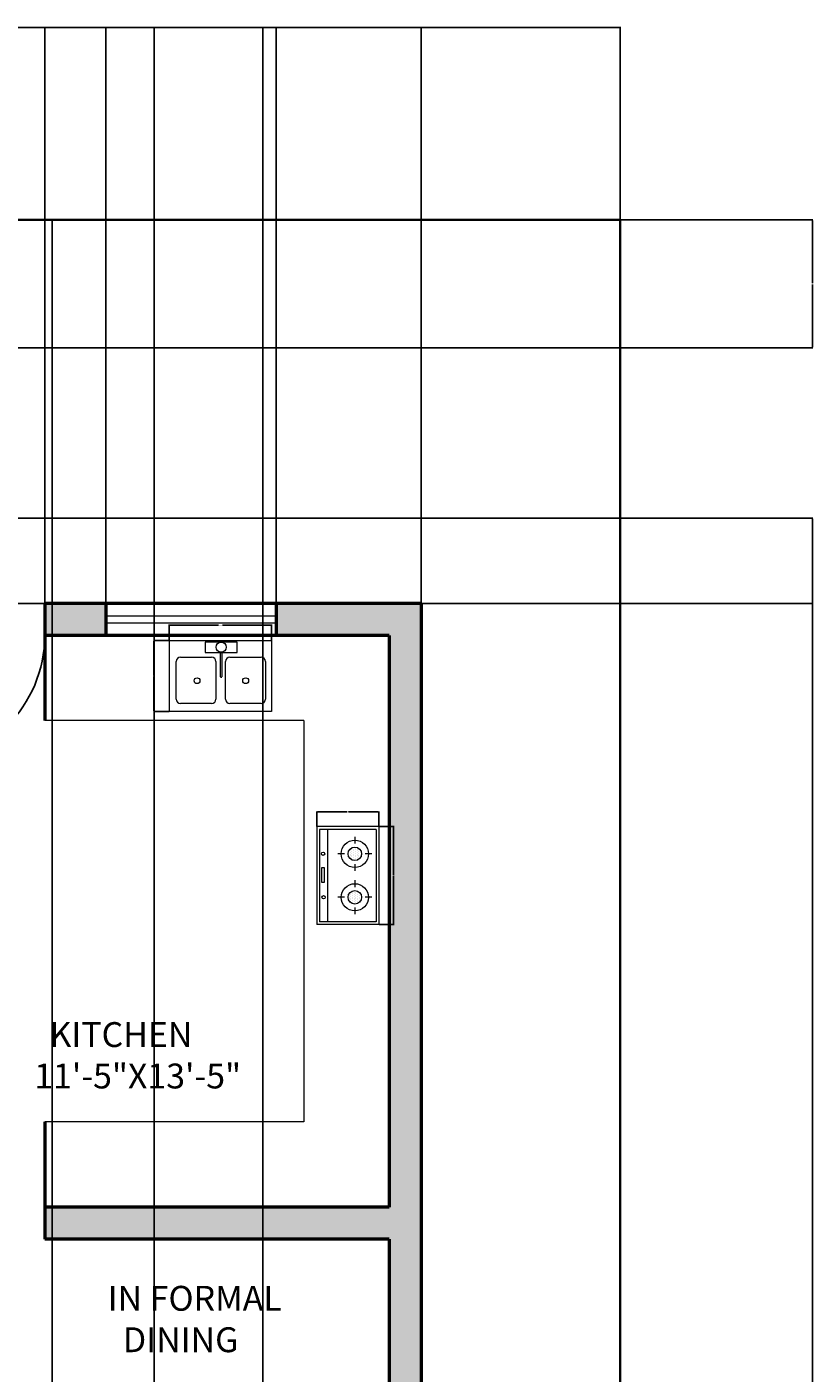
# Model space of a CAD drawing. Units: inches. Extents: x 2447 to 3157, y 2799 to 3988.
# Tile 9 of 9: x 2935 to 3157, y 3609 to 3988. Entities that reach past the tile are written whole.
import ezdxf

# ---------------------------------------------------------------- set-up
doc = ezdxf.new("R2010")
doc.units = ezdxf.units.IN
for name, color, linetype, lineweight in [('A-ANNO-DIMS', 2, 'Continuous', 18), ('A-AREA-IDEN', 7, 'Continuous', 25), ('A-DOOR', 3, 'Continuous', 25), ('A-EQPM', 8, 'Continuous', 18), ('A-FLOR-CASE', 8, 'Continuous', 20), ('A-FLOR-FIXT', 9, 'Continuous', 18), ('A-FLOR-STRS', 7, 'Continuous', 25), ('A-GLAZ', 4, 'Continuous', 18), ('A-WALL', 7, 'Continuous', 50), ('A-WALL-PATT', 252, 'Continuous', 13), ('C-PROP', 6, 'Continuous', 35)]:
    doc.layers.add(name, color=color, linetype=linetype, lineweight=lineweight)
doc.styles.get("Standard").update_dxf_attribs({"font": 'arial.ttf'})
doc.dimstyles.get("Standard").update_dxf_attribs({"dimtxt": 0.18, "dimasz": 0.18, "dimexe": 0.18, "dimexo": 0.0625, "dimgap": 0.09, "dimtad": 0, "dimtih": 1, "dimtoh": 1, "dimdec": 4, "dimzin": 0, "dimdsep": 46, "dimtxsty": 'Standard', "dimcen": 0.09, "dimadec": 0, "dimazin": 0, "dimtfac": 1, "dimtdec": 4, "dimtofl": 0, "dimtmove": 0, "dimatfit": 3, "dimfxl": 1, "dimtolj": 1, "dimtzin": 0, "dimarcsym": 0})

# ---------------------------------------------------------------- blocks, each defined once
blk = doc.blocks.new('A$C3AD04490')
for p, q in [((0, 641), (0, 0)), ((0, 641), (925, 641)), ((614, 627), (323, 627)), ((323, 627), (323, 532)), ((614, 532), (614, 627)), ((925, 641), (925, 0)), ((101, 490), (383, 490)), ((323, 532), (614, 532)), ((463, 312), (463, 537)), ((474, 537), (474, 312)), ((548, 490), (830, 490)), ((62, 111), (62, 451)), ((422, 451), (422, 111)), ((509, 111), (509, 451)), ((869, 451), (869, 111)), ((463, 311), (474, 311)), ((383, 72), (101, 72)), ((830, 72), (548, 72)), ((925, 0), (0, 0))]:
    blk.add_line(p, q)
for centre, radius in [((469, 581), 45.9), ((251, 278), 26.4), ((691, 278), 26.4)]:
    blk.add_circle(centre, radius)
for centre, start, end in [((101, 451), 90, 180), ((383, 451), 0, 90), ((548, 451), 90, 180), ((830, 451), 0, 90), ((101, 111), 180, 270), ((383, 111), 270, 0), ((548, 111), 180, 270), ((830, 111), 270, 0)]:
    blk.add_arc(centre, 39.1, start, end)
blk = doc.blocks.new('A$C475E21CF')
for p, q in [((0, 444.5), (0, 0)), ((0, 444.5), (699.9, 444.5)), ((19.4, 425), (19.4, 19.4)), ((19.4, 425), (680.5, 425)), ((194.5, 393.9), (194.5, 345.2)), ((505.4, 393.9), (505.4, 345.2)), ((680.5, 425), (680.5, 19.4)), ((699.9, 444.5), (699.9, 0)), ((166.9, 300.5), (166.9, 300.5)), ((179.1, 300.5), (179.1, 300.5)), ((185.2, 312.7), (185.2, 312.7)), ((191.2, 300.5), (191.2, 300.5)), ((197.3, 312.7), (197.3, 312.7)), ((203.4, 300.5), (203.4, 300.5)), ((209.5, 312.7), (209.5, 312.7)), ((215.6, 300.5), (215.6, 300.5)), ((227.7, 300.5), (227.7, 300.5)), ((474.1, 292.3), (474.1, 292.3)), ((480.2, 304.5), (480.2, 304.5)), ((486.3, 292.3), (486.3, 292.3)), ((492.3, 304.5), (492.3, 304.5)), ((498.4, 316.6), (498.4, 316.6)), ((498.4, 292.3), (498.4, 292.3)), ((504.5, 304.5), (504.5, 304.5)), ((510.6, 316.6), (510.6, 316.6)), ((510.6, 292.3), (510.6, 292.3)), ((516.7, 304.5), (516.7, 304.5)), ((522.7, 316.6), (522.7, 316.6)), ((522.7, 292.3), (522.7, 292.3)), ((528.8, 304.5), (528.8, 304.5)), ((534.9, 292.3), (534.9, 292.3)), ((541, 304.5), (541, 304.5)), ((547, 292.3), (547, 292.3)), ((72.9, 272.3), (121.6, 272.3)), ((148.7, 264.1), (148.7, 264.1)), ((154.8, 276.2), (154.8, 276.2)), ((154.8, 251.9), (154.8, 251.9)), ((160.9, 288.4), (160.9, 288.4)), ((160.9, 264.1), (160.9, 264.1)), ((160.9, 239.8), (160.9, 239.8)), ((166.9, 276.2), (166.9, 276.2)), ((166.9, 251.9), (166.9, 251.9)), ((173, 288.4), (173, 288.4)), ((173, 264.1), (173, 264.1)), ((173, 239.8), (173, 239.8)), ((179.1, 276.2), (179.1, 276.2)), ((179.1, 251.9), (179.1, 251.9)), ((179.1, 227.6), (179.1, 227.6)), ((185.2, 288.4), (185.2, 288.4)), ((185.2, 264.1), (185.2, 264.1)), ((185.2, 239.8), (185.2, 239.8)), ((191.2, 276.2), (191.2, 276.2)), ((191.2, 251.9), (191.2, 251.9)), ((191.2, 227.6), (191.2, 227.6)), ((194.5, 199.4), (194.5, 150.8)), ((197.3, 288.4), (197.3, 288.4)), ((197.3, 264.1), (197.3, 264.1)), ((197.3, 239.8), (197.3, 239.8)), ((203.4, 276.2), (203.4, 276.2)), ((203.4, 251.9), (203.4, 251.9)), ((203.4, 227.6), (203.4, 227.6)), ((209.5, 288.4), (209.5, 288.4)), ((209.5, 264.1), (209.5, 264.1)), ((209.5, 239.8), (209.5, 239.8)), ((215.6, 276.2), (215.6, 276.2)), ((215.6, 251.9), (215.6, 251.9)), ((215.6, 227.6), (215.6, 227.6)), ((221.6, 288.4), (221.6, 288.4)), ((221.6, 264.1), (221.6, 264.1)), ((221.6, 239.8), (221.6, 239.8)), ((227.7, 276.2), (227.7, 276.2)), ((227.7, 251.9), (227.7, 251.9)), ((233.8, 288.4), (233.8, 288.4)), ((233.8, 264.1), (233.8, 264.1)), ((233.8, 239.8), (233.8, 239.8)), ((239.9, 276.2), (239.9, 276.2)), ((239.9, 251.9), (239.9, 251.9)), ((267.4, 272.3), (316, 272.3)), ((383.9, 272.3), (432.5, 272.3)), ((462, 268), (462, 268)), ((468, 280.2), (468, 280.2)), ((468, 255.9), (468, 255.9)), ((474.1, 268), (474.1, 268)), ((474.1, 243.7), (474.1, 243.7)), ((480.2, 280.2), (480.2, 280.2)), ((480.2, 255.9), (480.2, 255.9)), ((486.3, 268), (486.3, 268)), ((486.3, 243.7), (486.3, 243.7)), ((492.3, 280.2), (492.3, 280.2)), ((492.3, 255.9), (492.3, 255.9)), ((492.3, 231.5), (492.3, 231.5)), ((498.4, 268), (498.4, 268)), ((498.4, 243.7), (498.4, 243.7)), ((504.5, 280.2), (504.5, 280.2)), ((504.5, 255.9), (504.5, 255.9)), ((504.5, 231.5), (504.5, 231.5)), ((505.4, 199.4), (505.4, 150.8)), ((510.6, 268), (510.6, 268)), ((510.6, 243.7), (510.6, 243.7)), ((516.7, 280.2), (516.7, 280.2)), ((516.7, 255.9), (516.7, 255.9)), ((516.7, 231.5), (516.7, 231.5)), ((522.7, 268), (522.7, 268)), ((522.7, 243.7), (522.7, 243.7)), ((528.8, 280.2), (528.8, 280.2)), ((528.8, 255.9), (528.8, 255.9)), ((528.8, 231.5), (528.8, 231.5)), ((534.9, 268), (534.9, 268)), ((534.9, 243.7), (534.9, 243.7)), ((541, 280.2), (541, 280.2)), ((541, 255.9), (541, 255.9)), ((547, 268), (547, 268)), ((547, 243.7), (547, 243.7)), ((553.1, 280.2), (553.1, 280.2)), ((553.1, 255.9), (553.1, 255.9)), ((578.4, 272.3), (627, 272.3)), ((0, 0), (699.9, 0)), ((19.4, 77.8), (680.5, 77.8)), ((19.4, 19.4), (680.5, 19.4)), ((293.4, 51.9), (400.6, 51.9)), ((293.4, 36.5), (293.4, 51.9)), ((400.6, 36.5), (293.4, 36.5)), ((400.6, 51.9), (400.6, 36.5))]:
    blk.add_line(p, q)
for centre, radius in [((194.5, 272.3), 97.2), ((194.5, 272.3), 48.6), ((505.4, 272.3), 97.2), ((505.4, 272.3), 48.6), ((193.9, 45.1), 11.7), ((505.2, 48.5), 11.7)]:
    blk.add_circle(centre, radius)
blk = doc.blocks.new('A$C1A936BB7')
blk.add_blockref('A$C475E21CF', (0, 0))
blk = doc.blocks.new('DOOR-SWING-36IN')
for p, q in [((0, 0), (0, 36)), ((1, 0), (1, 35.99)), ((1, 0), (0, 0))]:
    blk.add_line(p, q)
blk.add_arc((0, 0), 36, 0, 90)
blk = doc.blocks.new('*D30')
at = {"layer": 'A-ANNO-DIMS', "color": 0, "lineweight": -2, "transparency": 16777216}
for p, q in [((2975.45, 3815.28), (2975.45, 3819.71)), ((2975.63, 3819.53), (2989.29, 3819.53)), ((3004.04, 3819.53), (2990.38, 3819.53)), ((3004.22, 3815.28), (3004.22, 3819.71))]:
    blk.add_line(p, q, dxfattribs=at)
at = {"layer": 'A-ANNO-DIMS', "color": 0, "transparency": 16777216}
for points in [[(2975.63, 3819.56), (2975.63, 3819.5), (2975.45, 3819.53)], [(3004.04, 3819.56), (3004.04, 3819.5), (3004.22, 3819.53)]]:
    blk.add_solid(points, dxfattribs=at)
at = {"layer": 'Defpoints', "color": 0, "transparency": 16777216}
for p in [(3004.22, 3819.53), (2975.45, 3815.21), (3004.22, 3815.21)]:
    blk.add_point(p, dxfattribs=at)
at = {"layer": 'A-ANNO-DIMS', "color": 0, "transparency": 16777216, "insert": (2989.84, 3819.53), "char_height": 0.18, "attachment_point": 5}
blk.add_mtext('\\A1;SINK 29', dxfattribs=at)
blk = doc.blocks.new('*D31')
at = {"layer": 'A-ANNO-DIMS', "color": 0, "lineweight": -2, "transparency": 16777216}
for p, q in [((2975.39, 3815.21), (2970.95, 3815.21)), ((2971.13, 3815.03), (2971.13, 3805.43)), ((2971.13, 3795.46), (2971.13, 3805.07)), ((2975.39, 3795.28), (2970.95, 3795.28))]:
    blk.add_line(p, q, dxfattribs=at)
at = {"layer": 'A-ANNO-DIMS', "color": 0, "transparency": 16777216}
for points in [[(2971.1, 3815.03), (2971.16, 3815.03), (2971.13, 3815.21)], [(2971.1, 3795.46), (2971.16, 3795.46), (2971.13, 3795.28)]]:
    blk.add_solid(points, dxfattribs=at)
at = {"layer": 'Defpoints', "color": 0, "transparency": 16777216}
for p in [(2971.13, 3815.21), (2975.45, 3815.21), (2975.45, 3795.28)]:
    blk.add_point(p, dxfattribs=at)
at = {"layer": 'A-ANNO-DIMS', "color": 0, "transparency": 16777216, "insert": (2971.13, 3805.25), "char_height": 0.18, "attachment_point": 5}
blk.add_mtext('\\A1;20', dxfattribs=at)
blk = doc.blocks.new('*D32')
at = {"layer": 'A-ANNO-DIMS', "color": 0, "lineweight": -2, "transparency": 16777216}
for p, q in [((3034.53, 3762.83), (3038.78, 3762.83)), ((3038.6, 3762.65), (3038.6, 3749.24)), ((3038.6, 3735.46), (3038.6, 3748.87)), ((3034.53, 3735.28), (3038.78, 3735.28))]:
    blk.add_line(p, q, dxfattribs=at)
at = {"layer": 'A-ANNO-DIMS', "color": 0, "transparency": 16777216}
for points in [[(3038.57, 3762.65), (3038.63, 3762.65), (3038.6, 3762.83)], [(3038.57, 3735.46), (3038.63, 3735.46), (3038.6, 3735.28)]]:
    blk.add_solid(points, dxfattribs=at)
at = {"layer": 'Defpoints', "color": 0, "transparency": 16777216}
for p in [(3034.46, 3762.83), (3034.46, 3735.28), (3038.6, 3735.28)]:
    blk.add_point(p, dxfattribs=at)
at = {"layer": 'A-ANNO-DIMS', "color": 0, "transparency": 16777216, "insert": (3038.6, 3749.05), "char_height": 0.18, "attachment_point": 5}
blk.add_mtext('\\A1;HOB 28', dxfattribs=at)
blk = doc.blocks.new('*D33')
at = {"layer": 'A-ANNO-DIMS', "color": 0, "lineweight": -2, "transparency": 16777216}
for p, q in [((3016.96, 3762.89), (3016.96, 3767.14)), ((3017.14, 3766.96), (3025.5, 3766.96)), ((3034.28, 3766.96), (3025.92, 3766.96)), ((3034.46, 3762.89), (3034.46, 3767.14))]:
    blk.add_line(p, q, dxfattribs=at)
at = {"layer": 'A-ANNO-DIMS', "color": 0, "transparency": 16777216}
for points in [[(3017.14, 3766.99), (3017.14, 3766.93), (3016.96, 3766.96)], [(3034.28, 3766.99), (3034.28, 3766.93), (3034.46, 3766.96)]]:
    blk.add_solid(points, dxfattribs=at)
at = {"layer": 'Defpoints', "color": 0, "transparency": 16777216}
for p in [(3034.46, 3766.96), (3016.96, 3762.83), (3034.46, 3762.83)]:
    blk.add_point(p, dxfattribs=at)
at = {"layer": 'A-ANNO-DIMS', "color": 0, "transparency": 16777216, "insert": (3025.71, 3766.96), "char_height": 0.18, "attachment_point": 5}
blk.add_mtext('\\A1;17', dxfattribs=at)
blk = doc.blocks.new('*D46')
at = {"layer": 'A-ANNO-DIMS', "color": 0, "lineweight": -2, "transparency": 16777216}
for p, q in [((2561.37, 3849.76), (2561.37, 3988.03)), ((3046.37, 3825.76), (3046.37, 3988.03)), ((2561.55, 3987.85), (2803.57, 3987.85)), ((3046.19, 3987.85), (2804.16, 3987.85))]:
    blk.add_line(p, q, dxfattribs=at)
at = {"layer": 'A-ANNO-DIMS', "color": 0, "transparency": 16777216}
for points in [[(2561.55, 3987.88), (2561.55, 3987.82), (2561.37, 3987.85)], [(3046.19, 3987.88), (3046.19, 3987.82), (3046.37, 3987.85)]]:
    blk.add_solid(points, dxfattribs=at)
at = {"layer": 'Defpoints', "color": 0, "transparency": 16777216}
for p in [(3046.37, 3987.85), (2561.37, 3849.7), (3046.37, 3825.7)]:
    blk.add_point(p, dxfattribs=at)
at = {"layer": 'A-ANNO-DIMS', "color": 0, "transparency": 16777216, "insert": (2803.87, 3987.85), "char_height": 0.18, "attachment_point": 5}
blk.add_mtext('\\A1;485', dxfattribs=at)
blk = doc.blocks.new('*D47')
at = {"layer": 'A-ANNO-DIMS', "color": 0, "lineweight": -2, "transparency": 16777216}
for p, q in [((2798.43, 3849.7), (3156.7, 3849.7)), ((3156.52, 3849.52), (3156.52, 3487.38)), ((3156.52, 3124.88), (3156.52, 3487.02)), ((3046.43, 3124.7), (3156.7, 3124.7))]:
    blk.add_line(p, q, dxfattribs=at)
at = {"layer": 'A-ANNO-DIMS', "color": 0, "transparency": 16777216}
for points in [[(3156.49, 3849.52), (3156.55, 3849.52), (3156.52, 3849.7)], [(3156.49, 3124.88), (3156.55, 3124.88), (3156.52, 3124.7)]]:
    blk.add_solid(points, dxfattribs=at)
at = {"layer": 'Defpoints', "color": 0, "transparency": 16777216}
for p in [(2798.37, 3849.7), (3156.52, 3849.7), (3046.37, 3124.7)]:
    blk.add_point(p, dxfattribs=at)
at = {"layer": 'A-ANNO-DIMS', "color": 0, "transparency": 16777216, "insert": (3156.52, 3487.2), "char_height": 0.18, "attachment_point": 5}
blk.add_mtext('\\A1;725', dxfattribs=at)
blk = doc.blocks.new('*D49')
at = {"layer": 'A-ANNO-DIMS', "color": 0, "lineweight": -2, "transparency": 16777216}
for p, q in [((3046.37, 3825.76), (3046.37, 3988.03)), ((3102.37, 3933.76), (3102.37, 3988.03)), ((3046.55, 3987.85), (3074.15, 3987.85)), ((3102.19, 3987.85), (3074.59, 3987.85))]:
    blk.add_line(p, q, dxfattribs=at)
at = {"layer": 'A-ANNO-DIMS', "color": 0, "transparency": 16777216}
for points in [[(3046.55, 3987.88), (3046.55, 3987.82), (3046.37, 3987.85)], [(3102.19, 3987.88), (3102.19, 3987.82), (3102.37, 3987.85)]]:
    blk.add_solid(points, dxfattribs=at)
at = {"layer": 'Defpoints', "color": 0, "transparency": 16777216}
for p in [(3102.37, 3987.85), (3102.37, 3933.7), (3046.37, 3825.7)]:
    blk.add_point(p, dxfattribs=at)
at = {"layer": 'A-ANNO-DIMS', "color": 0, "transparency": 16777216, "insert": (3074.37, 3987.85), "char_height": 0.18, "attachment_point": 5}
blk.add_mtext('\\A1;56', dxfattribs=at)
blk = doc.blocks.new('*D50')
at = {"layer": 'A-ANNO-DIMS', "color": 0, "lineweight": -2, "transparency": 16777216}
for p, q in [((2832.46, 3897.64), (2832.46, 2799.37)), ((2942.46, 3897.64), (2942.46, 2799.37)), ((2832.64, 2799.55), (2887.18, 2799.55)), ((2942.28, 2799.55), (2887.74, 2799.55))]:
    blk.add_line(p, q, dxfattribs=at)
at = {"layer": 'A-ANNO-DIMS', "color": 0, "transparency": 16777216}
for points in [[(2832.64, 2799.58), (2832.64, 2799.52), (2832.46, 2799.55)], [(2942.28, 2799.58), (2942.28, 2799.52), (2942.46, 2799.55)]]:
    blk.add_solid(points, dxfattribs=at)
at = {"layer": 'Defpoints', "color": 0, "transparency": 16777216}
for p in [(2832.46, 3897.7), (2942.46, 3897.7), (2942.46, 2799.55)]:
    blk.add_point(p, dxfattribs=at)
at = {"layer": 'A-ANNO-DIMS', "color": 0, "transparency": 16777216, "insert": (2887.46, 2799.55), "char_height": 0.18, "attachment_point": 5}
blk.add_mtext('\\A1;110', dxfattribs=at)
blk = doc.blocks.new('*D51')
at = {"layer": 'A-ANNO-DIMS', "color": 0, "lineweight": -2, "transparency": 16777216}
for p, q in [((2942.52, 3933.7), (3156.7, 3933.7)), ((3156.52, 3933.52), (3156.52, 3915.88)), ((3156.52, 3897.88), (3156.52, 3915.52)), ((2942.52, 3897.7), (3156.7, 3897.7))]:
    blk.add_line(p, q, dxfattribs=at)
at = {"layer": 'A-ANNO-DIMS', "color": 0, "transparency": 16777216}
for points in [[(3156.49, 3933.52), (3156.55, 3933.52), (3156.52, 3933.7)], [(3156.49, 3897.88), (3156.55, 3897.88), (3156.52, 3897.7)]]:
    blk.add_solid(points, dxfattribs=at)
at = {"layer": 'Defpoints', "color": 0, "transparency": 16777216}
for p in [(2942.46, 3933.7), (3156.52, 3933.7), (2942.46, 3897.7)]:
    blk.add_point(p, dxfattribs=at)
at = {"layer": 'A-ANNO-DIMS', "color": 0, "transparency": 16777216, "insert": (3156.52, 3915.7), "char_height": 0.18, "attachment_point": 5}
blk.add_mtext('\\A1;36', dxfattribs=at)
blk = doc.blocks.new('*D62')
at = {"layer": 'A-ANNO-DIMS', "color": 0, "lineweight": -2, "transparency": 16777216}
for p, q in [((2798.43, 3849.7), (3156.7, 3849.7)), ((3156.52, 3849.52), (3156.52, 3837.88)), ((3156.52, 3825.88), (3156.52, 3837.52)), ((2798.43, 3825.7), (3156.7, 3825.7))]:
    blk.add_line(p, q, dxfattribs=at)
at = {"layer": 'A-ANNO-DIMS', "color": 0, "transparency": 16777216}
for points in [[(3156.49, 3849.52), (3156.55, 3849.52), (3156.52, 3849.7)], [(3156.49, 3825.88), (3156.55, 3825.88), (3156.52, 3825.7)]]:
    blk.add_solid(points, dxfattribs=at)
at = {"layer": 'Defpoints', "color": 0, "transparency": 16777216}
for p in [(2798.37, 3849.7), (2798.37, 3825.7), (3156.52, 3825.7)]:
    blk.add_point(p, dxfattribs=at)
at = {"layer": 'A-ANNO-DIMS', "color": 0, "transparency": 16777216, "insert": (3156.52, 3837.7), "char_height": 0.18, "attachment_point": 5}
blk.add_mtext('\\A1;24', dxfattribs=at)
blk = doc.blocks.new('*D65')
at = {"layer": 'A-ANNO-DIMS', "color": 0, "lineweight": -2, "transparency": 16777216}
for p, q in [((2940.37, 3825.76), (2940.37, 3988.03)), ((2957.58, 3825.76), (2957.58, 3988.03)), ((2940.55, 3987.85), (2948.52, 3987.85)), ((2957.4, 3987.85), (2949.43, 3987.85))]:
    blk.add_line(p, q, dxfattribs=at)
at = {"layer": 'A-ANNO-DIMS', "color": 0, "transparency": 16777216}
for points in [[(2940.55, 3987.88), (2940.55, 3987.82), (2940.37, 3987.85)], [(2957.4, 3987.88), (2957.4, 3987.82), (2957.58, 3987.85)]]:
    blk.add_solid(points, dxfattribs=at)
at = {"layer": 'Defpoints', "color": 0, "transparency": 16777216}
for p in [(2957.58, 3987.85), (2940.37, 3825.7), (2957.58, 3825.7)]:
    blk.add_point(p, dxfattribs=at)
at = {"layer": 'A-ANNO-DIMS', "color": 0, "transparency": 16777216, "insert": (2948.97, 3987.85), "char_height": 0.18, "attachment_point": 5}
blk.add_mtext('\\A1;17.213', dxfattribs=at)
blk = doc.blocks.new('*D66')
at = {"layer": 'A-ANNO-DIMS', "color": 0, "lineweight": -2, "transparency": 16777216}
for p, q in [((2957.58, 3825.76), (2957.58, 3988.03)), ((3005.58, 3825.76), (3005.58, 3988.03)), ((2957.76, 3987.85), (2981.36, 3987.85)), ((3005.4, 3987.85), (2981.8, 3987.85))]:
    blk.add_line(p, q, dxfattribs=at)
at = {"layer": 'A-ANNO-DIMS', "color": 0, "transparency": 16777216}
for points in [[(2957.76, 3987.88), (2957.76, 3987.82), (2957.58, 3987.85)], [(3005.4, 3987.88), (3005.4, 3987.82), (3005.58, 3987.85)]]:
    blk.add_solid(points, dxfattribs=at)
at = {"layer": 'Defpoints', "color": 0, "transparency": 16777216}
for p in [(3005.58, 3987.85), (2957.58, 3825.7), (3005.58, 3825.7)]:
    blk.add_point(p, dxfattribs=at)
at = {"layer": 'A-ANNO-DIMS', "color": 0, "transparency": 16777216, "insert": (2981.58, 3987.85), "char_height": 0.18, "attachment_point": 5}
blk.add_mtext('\\A1;48', dxfattribs=at)
blk = doc.blocks.new('*D67')
at = {"layer": 'A-ANNO-DIMS', "color": 0, "lineweight": -2, "transparency": 16777216}
for p, q in [((3005.58, 3825.76), (3005.58, 3988.03)), ((3046.37, 3825.76), (3046.37, 3988.03)), ((3005.76, 3987.85), (3025.58, 3987.85)), ((3046.19, 3987.85), (3026.37, 3987.85))]:
    blk.add_line(p, q, dxfattribs=at)
at = {"layer": 'A-ANNO-DIMS', "color": 0, "transparency": 16777216}
for points in [[(3005.76, 3987.88), (3005.76, 3987.82), (3005.58, 3987.85)], [(3046.19, 3987.88), (3046.19, 3987.82), (3046.37, 3987.85)]]:
    blk.add_solid(points, dxfattribs=at)
at = {"layer": 'Defpoints', "color": 0, "transparency": 16777216}
for p in [(3046.37, 3987.85), (3005.58, 3825.7), (3046.37, 3825.7)]:
    blk.add_point(p, dxfattribs=at)
at = {"layer": 'A-ANNO-DIMS', "color": 0, "transparency": 16777216, "insert": (3025.97, 3987.85), "char_height": 0.18, "attachment_point": 5}
blk.add_mtext('\\A1;40.79', dxfattribs=at)
blk = doc.blocks.new('*D70')
at = {"layer": 'A-ANNO-DIMS', "color": 0, "lineweight": -2, "transparency": 16777216}
for p, q in [((3001.81, 2980.76), (3001.81, 3988.03)), ((3102.37, 2853.76), (3102.37, 3988.03)), ((3001.99, 3987.85), (3051.63, 3987.85)), ((3102.19, 3987.85), (3052.54, 3987.85))]:
    blk.add_line(p, q, dxfattribs=at)
at = {"layer": 'A-ANNO-DIMS', "color": 0, "transparency": 16777216}
for points in [[(3001.99, 3987.88), (3001.99, 3987.82), (3001.81, 3987.85)], [(3102.19, 3987.88), (3102.19, 3987.82), (3102.37, 3987.85)]]:
    blk.add_solid(points, dxfattribs=at)
at = {"layer": 'Defpoints', "color": 0, "transparency": 16777216}
for p in [(3102.37, 3987.85), (3001.81, 2980.7), (3102.37, 2853.7)]:
    blk.add_point(p, dxfattribs=at)
at = {"layer": 'A-ANNO-DIMS', "color": 0, "transparency": 16777216, "insert": (3052.09, 3987.85), "char_height": 0.18, "attachment_point": 5}
blk.add_mtext('\\A1;100.56', dxfattribs=at)
blk = doc.blocks.new('*D76')
at = {"layer": 'A-ANNO-DIMS', "color": 0, "lineweight": -2, "transparency": 16777216}
for p, q in [((2847.64, 3124.76), (2847.64, 3988.03)), ((2971.17, 3124.76), (2971.17, 3988.03)), ((2847.82, 3987.85), (2908.95, 3987.85)), ((2970.99, 3987.85), (2909.86, 3987.85))]:
    blk.add_line(p, q, dxfattribs=at)
at = {"layer": 'A-ANNO-DIMS', "color": 0, "transparency": 16777216}
for points in [[(2847.82, 3987.88), (2847.82, 3987.82), (2847.64, 3987.85)], [(2970.99, 3987.88), (2970.99, 3987.82), (2971.17, 3987.85)]]:
    blk.add_solid(points, dxfattribs=at)
at = {"layer": 'Defpoints', "color": 0, "transparency": 16777216}
for p in [(2971.17, 3987.85), (2847.64, 3124.7), (2971.17, 3124.7)]:
    blk.add_point(p, dxfattribs=at)
at = {"layer": 'A-ANNO-DIMS', "color": 0, "transparency": 16777216, "insert": (2909.4, 3987.85), "char_height": 0.18, "attachment_point": 5}
blk.add_mtext('\\A1;123.53', dxfattribs=at)

msp = doc.modelspace()

# ---------------------------------------------------------------- hatches: boundary and pattern name
at = {"layer": 'A-WALL-PATT'}
h = msp.add_hatch(color=256, dxfattribs=at)
h.dxf.hatch_style = 1
h.paths.add_polyline_path([(2570.3672, 3550.7002), (2726.3672, 3550.7002), (2726.3672, 3370.7002), (2722.3672, 3370.7002), (2722.3672, 3365.7002), (2739.3672, 3365.7002), (2739.3672, 3374.7002), (2735.3672, 3374.7002), (2735.3672, 3563.7002), (2726.3672, 3563.7002), (2726.3672, 3559.7002), (2570.3672, 3559.7002), (2570.3672, 3599.2479), (2561.3672, 3599.2479), (2561.3672, 3508.7002), (2570.3672, 3508.7002)])
h.paths.add_polyline_path([(2570.3672, 3412.7002), (2561.3672, 3412.7002), (2561.3672, 3331.9279), (2570.3672, 3331.9279), (2570.3672, 3365.7002), (2666.3672, 3365.7002), (2666.3672, 3361.7002), (2671.3672, 3361.7002), (2671.3672, 3365.7002), (2686.3672, 3365.7002), (2686.3672, 3370.7002), (2570.3672, 3370.7002)])
h.paths.add_polyline_path([(2965.3672, 3430.7002), (2961.3672, 3430.7002), (2961.3672, 3434.7002), (2952.3672, 3434.7002), (2952.3672, 3430.7002), (2847.6393, 3430.7002), (2812.3672, 3395.4282), (2812.3672, 3374.7002), (2781.3672, 3374.7002), (2781.3672, 3365.7002), (2812.3672, 3365.7002), (2812.3672, 3347.7002), (2821.3672, 3347.7002), (2821.3672, 3391.7002), (2851.3672, 3421.7002), (2965.3672, 3421.7002)])
h.paths.add_polyline_path([(3046.3672, 3430.7002), (3033.3672, 3430.7002), (3033.3672, 3421.7002), (3037.3672, 3421.7002), (3037.3672, 3133.7002), (2971.1661, 3133.7002), (2971.1661, 3124.7002), (3046.3672, 3124.7002)])
h.paths.add_polyline_path([(3046.3672, 3825.7002), (3005.5801, 3825.7002), (3005.5801, 3816.7002), (3037.3672, 3816.7002), (3037.3672, 3655.7002), (2940.3672, 3655.7002), (2940.3672, 3646.7002), (3037.3672, 3646.7002), (3037.3672, 3514.7002), (3033.3672, 3514.7002), (3033.3672, 3505.7002), (3046.3672, 3505.7002)])
h.paths.add_polyline_path([(2821.3672, 3258.7002), (2812.3672, 3258.7002), (2812.3672, 3240.7002), (2808.3672, 3240.7002), (2808.3672, 3231.7002), (2812.3672, 3231.7002), (2812.3672, 3223.0688), (2821.3672, 3223.0688)])
h.paths.add_polyline_path([(2766.3672, 3240.7002), (2707.3672, 3240.7002), (2707.3672, 3234.4466, -1), (2570.3672, 3234.4466), (2570.3672, 3240.5271), (2561.3672, 3240.5271), (2561.3672, 3234.4466, 0.98243292), (2716.3185, 3231.7002), (2766.3672, 3231.7002)])
h.paths.add_polyline_path([(2570.3672, 3307.9279), (2561.3672, 3307.9279), (2561.3672, 3281.7773), (2570.3672, 3281.7773), (2570.3672, 3284.7002), (2671.3672, 3284.7002), (2671.3672, 3331.7002), (2666.3672, 3331.7002), (2666.3672, 3293.7002), (2570.3672, 3293.7002)])
h.paths.add_polyline_path([(2570.3672, 3739.7002), (2574.3672, 3739.7002), (2574.3672, 3744.7002), (2570.3672, 3744.7002), (2570.3672, 3840.7002), (2614.3672, 3840.7002), (2614.3672, 3849.7002), (2561.3672, 3849.7002), (2561.3672, 3671.2479), (2570.3672, 3671.2479)])
h.paths.add_polyline_path([(2735.3672, 3840.7002), (2789.3672, 3840.7002), (2789.3672, 3816.7002), (2798.3672, 3816.7002), (2798.3672, 3849.7002), (2679.3672, 3849.7002), (2679.3672, 3840.7002), (2726.3672, 3840.7002), (2726.3672, 3778.7002), (2735.3672, 3778.7002)])
h.paths.add_polyline_path([(2651.3672, 3840.7002), (2655.3672, 3840.7002), (2655.3672, 3849.7002), (2638.3672, 3849.7002), (2638.3672, 3840.7002), (2642.3672, 3840.7002), (2642.3672, 3744.7002), (2610.3672, 3744.7002), (2610.3672, 3739.7002), (2726.3672, 3739.7002), (2726.3672, 3599.7002), (2735.3672, 3599.7002), (2735.3672, 3622.7002), (2739.3672, 3622.7002), (2739.3672, 3631.7002), (2735.3672, 3631.7002), (2735.3672, 3748.7002), (2726.3672, 3748.7002), (2726.3672, 3744.7002), (2651.3672, 3744.7002)])
h.paths.add_polyline_path([(2900.3672, 3816.7002), (2904.3672, 3816.7002), (2904.3672, 3825.7002), (2882.3672, 3825.7002), (2882.3672, 3816.7002), (2891.3672, 3816.7002), (2891.3672, 3650.4282), (2872.6393, 3631.7002), (2775.3672, 3631.7002), (2775.3672, 3622.7002), (2876.3672, 3622.7002), (2900.3672, 3646.7002), (2904.3672, 3646.7002), (2904.3672, 3655.7002), (2900.3672, 3655.7002)])
h.paths.add_polyline_path([(2957.5801, 3825.7002), (2940.3672, 3825.7002), (2940.3672, 3816.7002), (2957.5801, 3816.7002)], flags=17)

# ---------------------------------------------------------------- linework, layer by layer
at = {"layer": 'A-FLOR-CASE'}
for p, q in [((3013.3672, 3792.7002), (2940.3672, 3792.7002)), ((3013.3672, 3792.7002), (3013.3672, 3679.7002)), ((3013.3672, 3679.7002), (2940.3672, 3679.7002))]:
    msp.add_line(p, q, dxfattribs=at)
at = {"layer": 'A-FLOR-STRS'}
for p, q in [((2942.456, 3897.7002), (2942.456, 3933.7002)), ((2832.456, 3897.7002), (2942.456, 3897.7002))]:
    msp.add_line(p, q, dxfattribs=at)
at = {"layer": 'A-GLAZ'}
for p, q in [((2957.5801, 3822.2002), (3005.5801, 3822.2002)), ((2957.5801, 3820.2002), (3005.5801, 3820.2002))]:
    msp.add_line(p, q, dxfattribs=at)
at = {"layer": 'A-WALL'}
for p, q in [((3046.3672, 3825.7002), (2940.3672, 3825.7002)), ((2940.3672, 3825.7002), (2940.3672, 3792.7002)), ((2957.5801, 3825.7002), (2957.5801, 3816.7002)), ((3005.5801, 3825.7002), (3005.5801, 3816.7002)), ((3046.3672, 3825.7002), (3046.3672, 3124.7002)), ((3037.3672, 3816.7002), (2940.3672, 3816.7002)), ((3037.3672, 3816.7002), (3037.3672, 3655.7002)), ((2940.3672, 3679.7002), (2940.3672, 3646.7002)), ((3037.3672, 3655.7002), (2940.3672, 3655.7002)), ((3037.3672, 3646.7002), (2940.3672, 3646.7002)), ((3037.3672, 3646.7002), (3037.3672, 3514.7002))]:
    msp.add_line(p, q, dxfattribs=at)
at = {"layer": 'C-PROP'}
for p, q in [((2501.3672, 3933.7002), (3102.3672, 3933.7002)), ((3102.3672, 3933.7002), (3102.3672, 2853.7002))]:
    msp.add_line(p, q, dxfattribs=at)

# ---------------------------------------------------------------- block references
at = {"layer": 'A-DOOR', "extrusion": (0, 0, -1), "zscale": -1, "rotation": 180}
msp.add_blockref('DOOR-SWING-36IN', (-2904.3672, 3816.7002), dxfattribs=at)
at = {"layer": 'A-EQPM', "xscale": 0.0393700787401575, "yscale": 0.0393700787401575, "zscale": 0.0393700787401575, "rotation": 270}
msp.add_blockref('A$C1A936BB7', (3016.9633, 3762.8312), dxfattribs=at)
at = {"layer": 'A-FLOR-FIXT', "xscale": 0.0311096401701662, "yscale": 0.0311096401701662, "zscale": 0.0311096401701662}
msp.add_blockref('A$C3AD04490', (2975.4506, 3795.2819), dxfattribs=at)

# ---------------------------------------------------------------- texts
at = {"layer": 'A-AREA-IDEN', "char_height": 7, "attachment_point": 1}
for s, width, insert in [('  KITCHEN\\P11\'-5"X13\'-5"', 62.074911, (2937.4049, 3707.778)), ('IN FORMAL\\P  DINING', 53.682608, (2958.0893, 3633.5097))]:
    msp.add_mtext_dynamic_manual_height_columns(s, width=width, gutter_width=12.5, heights=[0], dxfattribs=dict(at, insert=insert))

# ---------------------------------------------------------------- dimensions: what is measured, and where the dimension line sits
at = {"layer": 'A-ANNO-DIMS'}
for base, p1, p2, override, picture, middle in [((3046.3672, 3987.8502), (2561.3672, 3849.7002), (3046.3672, 3825.7002), {"dimdec": 0, "dimlfac": 1, "dimrnd": 0, "dimzin": 0, "dimdsep": 46, "dimlunit": 2}, '*D46', (2803.8672, 3987.8502)), ((2971.1661, 3987.8502), (2847.6393, 3124.7002), (2971.1661, 3124.7002), {"dimdec": 2, "dimlfac": 1, "dimrnd": 0, "dimzin": 0, "dimdsep": 46, "dimlunit": 2}, '*D76', (2909.4027, 3987.8502)), ((2957.5801, 3987.8502), (2940.3672, 3825.7002), (2957.5801, 3825.7002), {"dimdec": 3, "dimlfac": 1, "dimrnd": 0, "dimzin": 0, "dimdsep": 46, "dimlunit": 2}, '*D65', (2948.9737, 3987.8502)), ((3005.5801, 3987.8502), (2957.5801, 3825.7002), (3005.5801, 3825.7002), {"dimdec": 0, "dimlfac": 1, "dimrnd": 0, "dimzin": 0, "dimdsep": 46, "dimlunit": 2}, '*D66', (2981.5801, 3987.8502)), ((3102.3672, 3987.8502), (3001.807, 2980.7002), (3102.3672, 2853.7002), {"dimdec": 2, "dimlfac": 1, "dimrnd": 0, "dimzin": 0, "dimdsep": 46, "dimlunit": 2}, '*D70', (3052.0871, 3987.8502)), ((3046.3672, 3987.8502), (3005.5801, 3825.7002), (3046.3672, 3825.7002), {"dimdec": 2, "dimlfac": 1, "dimrnd": 0, "dimzin": 0, "dimdsep": 46, "dimlunit": 2}, '*D67', (3025.9737, 3987.8502)), ((3102.3672, 3987.8502), (3046.3672, 3825.7002), (3102.3672, 3933.7002), {"dimdec": 0, "dimlfac": 1, "dimrnd": 0, "dimzin": 0, "dimdsep": 46, "dimlunit": 2}, '*D49', (3074.3672, 3987.8502)), ((2942.456, 2799.5502), (2832.456, 3897.7002), (2942.456, 3897.7002), {"dimdec": 0, "dimlfac": 1, "dimrnd": 0, "dimzin": 0, "dimdsep": 46, "dimlunit": 2}, '*D50', (2887.456, 2799.5502)), ((3034.4631, 3766.9646), (3016.9633, 3762.8312), (3034.4631, 3762.8312), {"dimdec": 0, "dimlfac": 1, "dimrnd": 0, "dimzin": 0, "dimdsep": 46, "dimlunit": 2}, '*D33', (3025.7132, 3766.9646))]:
    dim = msp.add_linear_dim(base=base, p1=p1, p2=p2, dimstyle='Standard', override=override, dxfattribs=at)
    dim.commit()
    dim.dimension.update_dxf_attribs({"geometry": picture, "text_midpoint": middle})
for base, p1, p2, picture, middle in [((3156.5172, 3933.7002), (2942.456, 3897.7002), (2942.456, 3933.7002), '*D51', (3156.5172, 3915.7002)), ((3156.5172, 3849.7002), (3046.3672, 3124.7002), (2798.3672, 3849.7002), '*D47', (3156.5172, 3487.2002)), ((3156.5172, 3825.7002), (2798.3672, 3849.7002), (2798.3672, 3825.7002), '*D62', (3156.5172, 3837.7002)), ((2971.1345, 3815.215), (2975.4506, 3795.2819), (2975.4506, 3815.215), '*D31', (2971.1345, 3805.2485))]:
    dim = msp.add_linear_dim(base=base, p1=p1, p2=p2, angle=90, dimstyle='Standard', override={"dimdec": 0, "dimlfac": 1, "dimrnd": 0, "dimzin": 0, "dimdsep": 46, "dimlunit": 2}, dxfattribs=at)
    dim.commit()
    dim.dimension.update_dxf_attribs({"geometry": picture, "text_midpoint": middle})
dim = msp.add_linear_dim(base=(3004.2244, 3819.5311), p1=(2975.4506, 3815.215), p2=(3004.2244, 3815.215), text='SINK <>', dimstyle='Standard', override={"dimdec": 0, "dimlfac": 1, "dimrnd": 0, "dimzin": 0, "dimdsep": 46, "dimlunit": 2}, dxfattribs=at)
dim.commit()
dim.dimension.update_dxf_attribs({"geometry": '*D30', "text_midpoint": (2989.8375, 3819.5311)})
dim = msp.add_linear_dim(base=(3038.5965, 3735.2751), p1=(3034.4631, 3762.8312), p2=(3034.4631, 3735.2751), angle=270, text='HOB <>', dimstyle='Standard', override={"dimdec": 0, "dimlfac": 1, "dimrnd": 0, "dimzin": 0, "dimdsep": 46, "dimlunit": 2}, dxfattribs=at)
dim.commit()
dim.dimension.update_dxf_attribs({"geometry": '*D32', "text_midpoint": (3038.5965, 3749.0531)})

doc.saveas('drawing.dxf')
